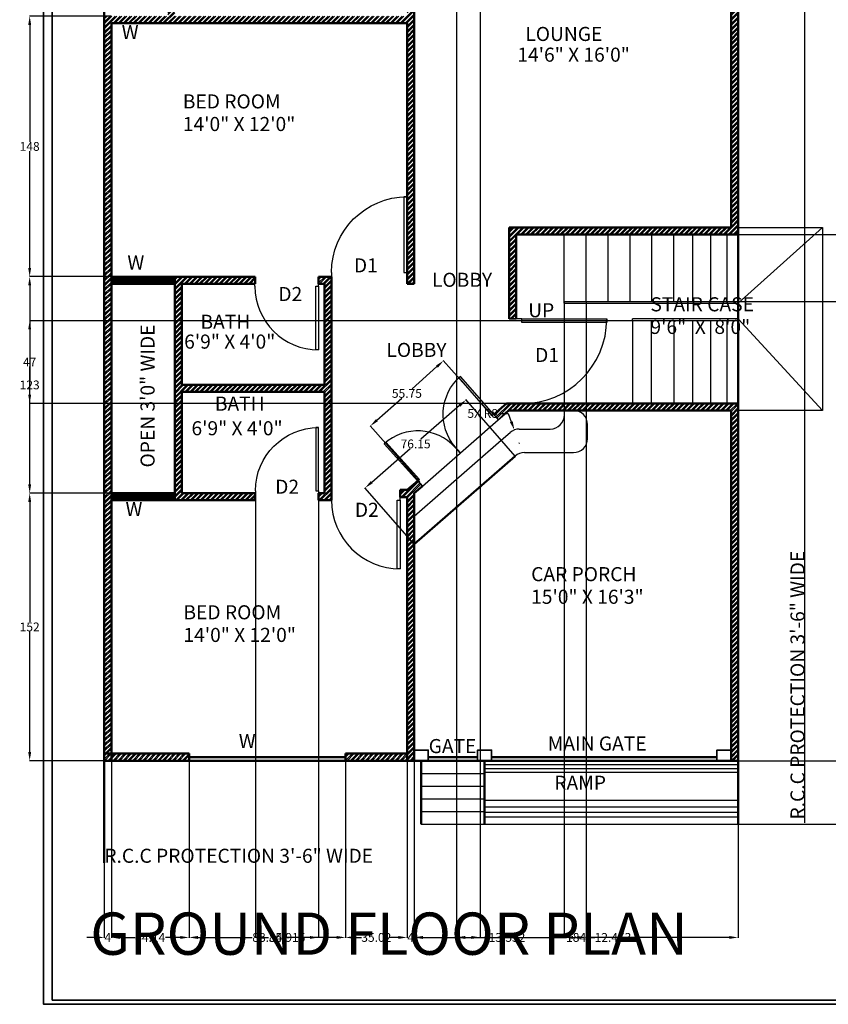
# Model space of a CAD drawing. Units: inches. Extents: x -35 to 905, y -602 to 298.
# Tile 1 of 4: x -30 to 429, y -602 to -43. Entities that reach past the tile are written whole.
import ezdxf

# ---------------------------------------------------------------- set-up
doc = ezdxf.new("R2010")
doc.units = ezdxf.units.IN
doc.header["$MEASUREMENT"] = 0
for name, color, linetype, lineweight in [('A-ANNO-DIMS', 2, 'Continuous', 18), ('A-ANNO-TEXT', 3, 'Continuous', 18), ('A-ANNO-TTLB', 7, 'Continuous', 35), ('A-AREA-IDEN', 7, 'Continuous', 18), ('A-COLS', 7, 'Continuous', 35), ('A-DOOR', 4, 'Continuous', 25), ('A-FLOR-STRS', 3, 'Continuous', 25), ('A-WALL', 7, 'Continuous', 50), ('A-WALL-PATT', 8, 'Continuous', 13), ('C-PROP', 1, 'Continuous', 25)]:
    doc.layers.add(name, color=color, linetype=linetype, lineweight=lineweight)
doc.styles.get("Standard").update_dxf_attribs({"font": 'arial.ttf'})
doc.dimstyles.get("Standard").update_dxf_attribs({"dimtxt": 5, "dimasz": 5, "dimexe": 0.18, "dimexo": 0.0625, "dimgap": 0.09, "dimtad": 0, "dimtih": 1, "dimtoh": 1, "dimdec": 1, "dimzin": 0, "dimdsep": 46, "dimlunit": 4, "dimtxsty": 'Standard', "dimcen": 0.09, "dimadec": 0, "dimazin": 0, "dimtfac": 1, "dimtdec": 1, "dimtofl": 0, "dimtmove": 0, "dimatfit": 3, "dimfxl": 1, "dimtolj": 1, "dimtzin": 0, "dimarcsym": 0})

# ---------------------------------------------------------------- blocks, each defined once
blk = doc.blocks.new('*U2')
for p, q in [((0, 0), (0, -6)), ((40, 0), (40, -6))]:
    blk.add_line(p, q)
blk.add_lwpolyline([(0, 0), (0, 40), (1.75, 40), (1.75, 0)], close=True)
blk.add_arc((0, 0), 40, 0, 90)
blk = doc.blocks.new('*D8')
at = {"layer": 'A-ANNO-DIMS', "color": 0, "lineweight": -2, "ltscale": 0.3, "transparency": 16777216}
for p, q in [((21.72, -40.65), (-24.8, -40.65)), ((-24.62, -45.65), (-24.62, -112.01)), ((-24.62, -183.65), (-24.62, -117.3)), ((21.72, -188.65), (-24.8, -188.65))]:
    blk.add_line(p, q, dxfattribs=at)
at = {"layer": 'A-ANNO-DIMS', "color": 0, "ltscale": 0.3, "transparency": 16777216}
for points in [[(-25.45, -45.65), (-23.78, -45.65), (-24.62, -40.65)], [(-25.45, -183.65), (-23.78, -183.65), (-24.62, -188.65)]]:
    blk.add_solid(points, dxfattribs=at)
at = {"layer": 'Defpoints', "color": 0, "ltscale": 0.3, "transparency": 16777216}
for p in [(21.78, -40.65), (-24.62, -188.65), (21.78, -188.65)]:
    blk.add_point(p, dxfattribs=at)
at = {"layer": 'A-ANNO-DIMS', "color": 0, "ltscale": 0.3, "transparency": 16777216, "insert": (-24.62, -114.65), "char_height": 5, "attachment_point": 5}
blk.add_mtext('\\A1;148', dxfattribs=at)
blk = doc.blocks.new('*D9')
at = {"layer": 'A-ANNO-DIMS', "color": 0, "lineweight": -2, "ltscale": 0.3, "transparency": 16777216}
for p, q in [((21.72, -188.65), (-24.8, -188.65)), ((-24.62, -193.65), (-24.62, -247.51)), ((-24.62, -306.65), (-24.62, -252.8)), ((21.72, -311.65), (-24.8, -311.65))]:
    blk.add_line(p, q, dxfattribs=at)
at = {"layer": 'A-ANNO-DIMS', "color": 0, "ltscale": 0.3, "transparency": 16777216}
for points in [[(-25.45, -193.65), (-23.78, -193.65), (-24.62, -188.65)], [(-25.45, -306.65), (-23.78, -306.65), (-24.62, -311.65)]]:
    blk.add_solid(points, dxfattribs=at)
at = {"layer": 'Defpoints', "color": 0, "ltscale": 0.3, "transparency": 16777216}
for p in [(21.78, -188.65), (-24.62, -311.65), (21.78, -311.65)]:
    blk.add_point(p, dxfattribs=at)
at = {"layer": 'A-ANNO-DIMS', "color": 0, "ltscale": 0.3, "transparency": 16777216, "insert": (-24.62, -250.15), "char_height": 5, "attachment_point": 5}
blk.add_mtext('\\A1;123', dxfattribs=at)
blk = doc.blocks.new('*D10')
at = {"layer": 'A-ANNO-DIMS', "color": 0, "lineweight": -2, "ltscale": 0.3, "transparency": 16777216}
for p, q in [((21.72, -311.65), (-24.8, -311.65)), ((-24.62, -316.65), (-24.62, -385.01)), ((-24.62, -458.65), (-24.62, -390.3)), ((17.72, -463.65), (-24.8, -463.65))]:
    blk.add_line(p, q, dxfattribs=at)
at = {"layer": 'A-ANNO-DIMS', "color": 0, "ltscale": 0.3, "transparency": 16777216}
for points in [[(-25.45, -316.65), (-23.78, -316.65), (-24.62, -311.65)], [(-25.45, -458.65), (-23.78, -458.65), (-24.62, -463.65)]]:
    blk.add_solid(points, dxfattribs=at)
at = {"layer": 'Defpoints', "color": 0, "ltscale": 0.3, "transparency": 16777216}
for p in [(21.78, -311.65), (-24.62, -463.65), (17.78, -463.65)]:
    blk.add_point(p, dxfattribs=at)
at = {"layer": 'A-ANNO-DIMS', "color": 0, "ltscale": 0.3, "transparency": 16777216, "insert": (-24.62, -387.65), "char_height": 5, "attachment_point": 5}
blk.add_mtext('\\A1;152', dxfattribs=at)
blk = doc.blocks.new('*D11')
at = {"layer": 'A-ANNO-DIMS', "color": 0, "lineweight": -2, "ltscale": 0.3, "transparency": 16777216}
for p, q in [((17.78, -463.72), (17.78, -564.24)), ((21.78, -463.72), (21.78, -564.24)), ((12.78, -564.06), (7.78, -564.06)), ((26.78, -564.06), (31.78, -564.06))]:
    blk.add_line(p, q, dxfattribs=at)
at = {"layer": 'A-ANNO-DIMS', "color": 0, "ltscale": 0.3, "transparency": 16777216}
for points in [[(12.78, -563.23), (12.78, -564.9), (17.78, -564.06)], [(26.78, -563.23), (26.78, -564.9), (21.78, -564.06)]]:
    blk.add_solid(points, dxfattribs=at)
at = {"layer": 'Defpoints', "color": 0, "ltscale": 0.3, "transparency": 16777216}
for p in [(17.78, -463.65), (21.78, -463.65), (21.78, -564.06)]:
    blk.add_point(p, dxfattribs=at)
at = {"layer": 'A-ANNO-DIMS', "color": 0, "ltscale": 0.3, "transparency": 16777216, "insert": (19.78, -564.06), "char_height": 5, "attachment_point": 5}
blk.add_mtext('\\A1;4', dxfattribs=at)
blk = doc.blocks.new('*D12')
at = {"layer": 'A-ANNO-DIMS', "color": 0, "lineweight": -2, "ltscale": 0.3, "transparency": 16777216}
for p, q in [((21.78, -463.72), (21.78, -564.24)), ((65.92, -459.72), (65.92, -564.24)), ((26.78, -564.06), (35.24, -564.06)), ((60.92, -564.06), (52.47, -564.06))]:
    blk.add_line(p, q, dxfattribs=at)
at = {"layer": 'A-ANNO-DIMS', "color": 0, "ltscale": 0.3, "transparency": 16777216}
for points in [[(26.78, -563.23), (26.78, -564.9), (21.78, -564.06)], [(60.92, -563.23), (60.92, -564.9), (65.92, -564.06)]]:
    blk.add_solid(points, dxfattribs=at)
at = {"layer": 'Defpoints', "color": 0, "ltscale": 0.3, "transparency": 16777216}
for p in [(21.78, -463.65), (65.92, -459.65), (65.92, -564.06)]:
    blk.add_point(p, dxfattribs=at)
at = {"layer": 'A-ANNO-DIMS', "color": 0, "ltscale": 0.3, "transparency": 16777216, "insert": (43.85, -564.06), "char_height": 5, "attachment_point": 5}
blk.add_mtext('\\A1;44.14', dxfattribs=at)
blk = doc.blocks.new('*D13')
at = {"layer": 'A-ANNO-DIMS', "color": 0, "lineweight": -2, "ltscale": 0.3, "transparency": 16777216}
for p, q in [((65.92, -459.72), (65.92, -564.24)), ((154.77, -459.72), (154.77, -564.24)), ((70.92, -564.06), (101.83, -564.06)), ((149.77, -564.06), (118.86, -564.06))]:
    blk.add_line(p, q, dxfattribs=at)
at = {"layer": 'A-ANNO-DIMS', "color": 0, "ltscale": 0.3, "transparency": 16777216}
for points in [[(70.92, -563.23), (70.92, -564.9), (65.92, -564.06)], [(149.77, -563.23), (149.77, -564.9), (154.77, -564.06)]]:
    blk.add_solid(points, dxfattribs=at)
at = {"layer": 'Defpoints', "color": 0, "ltscale": 0.3, "transparency": 16777216}
for p in [(65.92, -459.65), (154.77, -459.65), (154.77, -564.06)]:
    blk.add_point(p, dxfattribs=at)
at = {"layer": 'A-ANNO-DIMS', "color": 0, "ltscale": 0.3, "transparency": 16777216, "insert": (110.35, -564.06), "char_height": 5, "attachment_point": 5}
blk.add_mtext('\\A1;88.84', dxfattribs=at)
blk = doc.blocks.new('*D14')
at = {"layer": 'A-ANNO-DIMS', "color": 0, "lineweight": -2, "ltscale": 0.3, "transparency": 16777216}
for p, q in [((154.77, -459.72), (154.77, -564.24)), ((189.78, -459.72), (189.78, -564.24)), ((159.77, -564.06), (163.78, -564.06)), ((184.78, -564.06), (180.77, -564.06))]:
    blk.add_line(p, q, dxfattribs=at)
at = {"layer": 'A-ANNO-DIMS', "color": 0, "ltscale": 0.3, "transparency": 16777216}
for points in [[(159.77, -563.23), (159.77, -564.9), (154.77, -564.06)], [(184.78, -563.23), (184.78, -564.9), (189.78, -564.06)]]:
    blk.add_solid(points, dxfattribs=at)
at = {"layer": 'Defpoints', "color": 0, "ltscale": 0.3, "transparency": 16777216}
for p in [(154.77, -459.65), (189.78, -459.65), (189.78, -564.06)]:
    blk.add_point(p, dxfattribs=at)
at = {"layer": 'A-ANNO-DIMS', "color": 0, "ltscale": 0.3, "transparency": 16777216, "insert": (172.28, -564.06), "char_height": 5, "attachment_point": 5}
blk.add_mtext('\\A1;35.02', dxfattribs=at)
blk = doc.blocks.new('*D15')
at = {"layer": 'A-ANNO-DIMS', "color": 0, "lineweight": -2, "ltscale": 0.3, "transparency": 16777216}
for p, q in [((193.78, -457.67), (193.78, -564.24)), ((189.78, -459.72), (189.78, -564.24)), ((184.78, -564.06), (179.78, -564.06)), ((198.78, -564.06), (203.78, -564.06))]:
    blk.add_line(p, q, dxfattribs=at)
at = {"layer": 'A-ANNO-DIMS', "color": 0, "ltscale": 0.3, "transparency": 16777216}
for points in [[(184.78, -563.23), (184.78, -564.9), (189.78, -564.06)], [(198.78, -563.23), (198.78, -564.9), (193.78, -564.06)]]:
    blk.add_solid(points, dxfattribs=at)
at = {"layer": 'Defpoints', "color": 0, "ltscale": 0.3, "transparency": 16777216}
for p in [(193.78, -457.61), (189.78, -459.65), (193.78, -564.06)]:
    blk.add_point(p, dxfattribs=at)
at = {"layer": 'A-ANNO-DIMS', "color": 0, "ltscale": 0.3, "transparency": 16777216, "insert": (191.78, -564.06), "char_height": 5, "attachment_point": 5}
blk.add_mtext('\\A1;4', dxfattribs=at)
blk = doc.blocks.new('*D16')
at = {"layer": 'A-ANNO-DIMS', "color": 0, "lineweight": -2, "ltscale": 0.3, "transparency": 16777216}
for p, q in [((193.78, -457.67), (193.78, -564.24)), ((377.78, -463.72), (377.78, -564.24)), ((198.78, -564.06), (280.42, -564.06)), ((372.78, -564.06), (291.15, -564.06))]:
    blk.add_line(p, q, dxfattribs=at)
at = {"layer": 'A-ANNO-DIMS', "color": 0, "ltscale": 0.3, "transparency": 16777216}
for points in [[(198.78, -563.23), (198.78, -564.9), (193.78, -564.06)], [(372.78, -563.23), (372.78, -564.9), (377.78, -564.06)]]:
    blk.add_solid(points, dxfattribs=at)
at = {"layer": 'Defpoints', "color": 0, "ltscale": 0.3, "transparency": 16777216}
for p in [(193.78, -457.61), (377.78, -463.65), (377.78, -564.06)]:
    blk.add_point(p, dxfattribs=at)
at = {"layer": 'A-ANNO-DIMS', "color": 0, "ltscale": 0.3, "transparency": 16777216, "insert": (285.78, -564.06), "char_height": 5, "attachment_point": 5}
blk.add_mtext('\\A1;184', dxfattribs=at)
blk = doc.blocks.new('*D17')
at = {"layer": 'A-ANNO-DIMS', "color": 0, "lineweight": -2, "ltscale": 0.3, "transparency": 16777216}
for p, q in [((377.85, -463.65), (468.36, -463.65)), ((468.18, -468.65), (468.18, -479.01)), ((468.18, -494.65), (468.18, -484.3)), ((377.85, -499.65), (468.36, -499.65))]:
    blk.add_line(p, q, dxfattribs=at)
at = {"layer": 'A-ANNO-DIMS', "color": 0, "ltscale": 0.3, "transparency": 16777216}
for points in [[(467.35, -468.65), (469.02, -468.65), (468.18, -463.65)], [(467.35, -494.65), (469.02, -494.65), (468.18, -499.65)]]:
    blk.add_solid(points, dxfattribs=at)
at = {"layer": 'Defpoints', "color": 0, "ltscale": 0.3, "transparency": 16777216}
for p in [(377.78, -463.65), (377.78, -499.65), (468.18, -499.65)]:
    blk.add_point(p, dxfattribs=at)
at = {"layer": 'A-ANNO-DIMS', "color": 0, "ltscale": 0.3, "transparency": 16777216, "insert": (468.18, -481.65), "char_height": 5, "attachment_point": 5}
blk.add_mtext('\\A1;36', dxfattribs=at)
blk = doc.blocks.new('*D18')
at = {"layer": 'A-ANNO-DIMS', "color": 0, "lineweight": -2, "ltscale": 0.3, "transparency": 16777216}
for p, q in [((377.85, 249.35), (468.36, 249.35)), ((468.18, 244.35), (468.18, -104.51)), ((468.18, -458.65), (468.18, -109.8)), ((377.85, -463.65), (468.36, -463.65))]:
    blk.add_line(p, q, dxfattribs=at)
at = {"layer": 'A-ANNO-DIMS', "color": 0, "ltscale": 0.3, "transparency": 16777216}
for points in [[(467.35, 244.35), (469.02, 244.35), (468.18, 249.35)], [(467.35, -458.65), (469.02, -458.65), (468.18, -463.65)]]:
    blk.add_solid(points, dxfattribs=at)
at = {"layer": 'Defpoints', "color": 0, "ltscale": 0.3, "transparency": 16777216}
for p in [(377.78, 249.35), (377.78, -463.65), (468.18, -463.65)]:
    blk.add_point(p, dxfattribs=at)
at = {"layer": 'A-ANNO-DIMS', "color": 0, "ltscale": 0.3, "transparency": 16777216, "insert": (468.18, -107.15), "char_height": 5, "attachment_point": 5}
blk.add_mtext('\\A1;713', dxfattribs=at)
blk = doc.blocks.new('*D21')
at = {"layer": 'A-ANNO-DIMS', "color": 0, "lineweight": -2, "ltscale": 0.3, "transparency": 16777216}
for p, q in [((103.62, -315.72), (103.62, -564.24)), ((139.54, -315.72), (139.54, -564.24)), ((108.62, -564.06), (111.09, -564.06)), ((134.54, -564.06), (132.07, -564.06))]:
    blk.add_line(p, q, dxfattribs=at)
at = {"layer": 'A-ANNO-DIMS', "color": 0, "ltscale": 0.3, "transparency": 16777216}
for points in [[(108.62, -563.23), (108.62, -564.9), (103.62, -564.06)], [(134.54, -563.23), (134.54, -564.9), (139.54, -564.06)]]:
    blk.add_solid(points, dxfattribs=at)
at = {"layer": 'Defpoints', "color": 0, "ltscale": 0.3, "transparency": 16777216}
for p in [(103.62, -315.65), (139.54, -315.65), (139.54, -564.06)]:
    blk.add_point(p, dxfattribs=at)
at = {"layer": 'A-ANNO-DIMS', "color": 0, "ltscale": 0.3, "transparency": 16777216, "insert": (121.58, -564.06), "char_height": 5, "attachment_point": 5}
blk.add_mtext('\\A1;35.915', dxfattribs=at)
blk = doc.blocks.new('*D24')
at = {"layer": 'A-ANNO-DIMS', "color": 0, "lineweight": -2, "ltscale": 0.3, "transparency": 16777216}
for p, q in [((206.74, -239.75), (192.62, -252.35)), ((238.65, -268.02), (210.35, -236.29)), ((172.6, -270.21), (186.72, -257.61)), ((197.05, -305.13), (168.75, -273.4))]:
    blk.add_line(p, q, dxfattribs=at)
at = {"layer": 'A-ANNO-DIMS', "color": 0, "ltscale": 0.3, "transparency": 16777216}
for points in [[(206.18, -239.13), (207.29, -240.37), (210.47, -236.42)], [(172.05, -269.58), (173.16, -270.83), (168.87, -273.54)]]:
    blk.add_solid(points, dxfattribs=at)
at = {"layer": 'Defpoints', "color": 0, "ltscale": 0.3, "transparency": 16777216}
for p in [(210.47, -236.42), (238.7, -268.06), (197.1, -305.17)]:
    blk.add_point(p, dxfattribs=at)
at = {"layer": 'A-ANNO-DIMS', "color": 0, "ltscale": 0.3, "transparency": 16777216, "insert": (189.67, -254.98), "char_height": 5, "attachment_point": 5}
blk.add_mtext('\\A1;55.75', dxfattribs=at)
blk = doc.blocks.new('*D25')
at = {"layer": 'A-ANNO-DIMS', "color": 0, "lineweight": -2, "ltscale": 0.3, "transparency": 16777216}
for p, q in [((217.78, 218.55), (217.78, -564.24)), ((231.32, 218.55), (231.32, -564.24)), ((222.78, -564.06), (226.32, -564.06)), ((231.32, -564.06), (236.32, -564.06))]:
    blk.add_line(p, q, dxfattribs=at)
at = {"layer": 'A-ANNO-DIMS', "color": 0, "ltscale": 0.3, "transparency": 16777216}
for points in [[(222.78, -563.23), (222.78, -564.9), (217.78, -564.06)], [(226.32, -563.23), (226.32, -564.9), (231.32, -564.06)]]:
    blk.add_solid(points, dxfattribs=at)
at = {"layer": 'Defpoints', "color": 0, "ltscale": 0.3, "transparency": 16777216}
for p in [(217.78, 218.61), (231.32, 218.61), (231.32, -564.06)]:
    blk.add_point(p, dxfattribs=at)
at = {"layer": 'A-ANNO-DIMS', "color": 0, "ltscale": 0.3, "transparency": 16777216, "insert": (246.52, -564.06), "char_height": 5, "attachment_point": 5}
blk.add_mtext('\\A1;13.532', dxfattribs=at)
blk = doc.blocks.new('*D27')
at = {"layer": 'A-ANNO-DIMS', "color": 0, "lineweight": -2, "ltscale": 0.3, "transparency": 16777216}
for p, q in [((279.03, -202.74), (279.03, -564.24)), ((291.5, -202.74), (291.5, -564.24)), ((284.03, -564.06), (286.5, -564.06)), ((291.5, -564.06), (296.5, -564.06))]:
    blk.add_line(p, q, dxfattribs=at)
at = {"layer": 'A-ANNO-DIMS', "color": 0, "ltscale": 0.3, "transparency": 16777216}
for points in [[(284.03, -563.23), (284.03, -564.9), (279.03, -564.06)], [(286.5, -563.23), (286.5, -564.9), (291.5, -564.06)]]:
    blk.add_solid(points, dxfattribs=at)
at = {"layer": 'Defpoints', "color": 0, "ltscale": 0.3, "transparency": 16777216}
for p in [(279.03, -202.67), (291.5, -202.67), (291.5, -564.06)]:
    blk.add_point(p, dxfattribs=at)
at = {"layer": 'A-ANNO-DIMS', "color": 0, "ltscale": 0.3, "transparency": 16777216, "insert": (306.73, -564.06), "char_height": 5, "attachment_point": 5}
blk.add_mtext('\\A1;12.463', dxfattribs=at)
blk = doc.blocks.new('*D28')
at = {"layer": 'A-ANNO-DIMS', "color": 0, "lineweight": -2, "ltscale": 0.3, "transparency": 16777216}
for p, q in [((279.1, -164.65), (468.36, -164.65)), ((468.18, -169.65), (468.18, -181.02)), ((468.18, -197.67), (468.18, -186.31)), ((279.1, -202.67), (468.36, -202.67))]:
    blk.add_line(p, q, dxfattribs=at)
at = {"layer": 'A-ANNO-DIMS', "color": 0, "ltscale": 0.3, "transparency": 16777216}
for points in [[(467.35, -169.65), (469.02, -169.65), (468.18, -164.65)], [(467.35, -197.67), (469.02, -197.67), (468.18, -202.67)]]:
    blk.add_solid(points, dxfattribs=at)
at = {"layer": 'Defpoints', "color": 0, "ltscale": 0.3, "transparency": 16777216}
for p in [(279.03, -164.65), (279.03, -202.67), (468.18, -202.67)]:
    blk.add_point(p, dxfattribs=at)
at = {"layer": 'A-ANNO-DIMS', "color": 0, "ltscale": 0.3, "transparency": 16777216, "insert": (468.18, -183.66), "char_height": 5, "attachment_point": 5}
blk.add_mtext('\\A1;38.02', dxfattribs=at)
blk = doc.blocks.new('*D29')
at = {"layer": 'A-ANNO-DIMS', "color": 0, "lineweight": -2, "ltscale": 0.3, "transparency": 16777216}
for p, q in [((317.72, -213.65), (-24.8, -213.65)), ((-24.62, -218.65), (-24.62, -234.56)), ((-24.62, -255.65), (-24.62, -239.74)), ((317.72, -260.65), (-24.8, -260.65))]:
    blk.add_line(p, q, dxfattribs=at)
at = {"layer": 'A-ANNO-DIMS', "color": 0, "ltscale": 0.3, "transparency": 16777216}
for points in [[(-25.45, -218.65), (-23.78, -218.65), (-24.62, -213.65)], [(-25.45, -255.65), (-23.78, -255.65), (-24.62, -260.65)]]:
    blk.add_solid(points, dxfattribs=at)
at = {"layer": 'Defpoints', "color": 0, "ltscale": 0.3, "transparency": 16777216}
for p in [(317.78, -213.65), (-24.62, -260.65), (317.78, -260.65)]:
    blk.add_point(p, dxfattribs=at)
at = {"layer": 'A-ANNO-DIMS', "color": 0, "ltscale": 0.3, "transparency": 16777216, "insert": (-24.62, -237.15), "char_height": 5, "attachment_point": 5}
blk.add_mtext('\\A1;47', dxfattribs=at)
blk = doc.blocks.new('*D30')
at = {"layer": 'A-ANNO-DIMS', "color": 0, "lineweight": -2, "ltscale": 0.3, "transparency": 16777216}
for p, q in [((219.53, -261.92), (197.63, -281.03)), ((251.13, -290.54), (223.18, -258.5)), ((169.68, -305.41), (191.57, -286.31)), ((193.74, -340.6), (165.79, -308.57))]:
    blk.add_line(p, q, dxfattribs=at)
at = {"layer": 'A-ANNO-DIMS', "color": 0, "ltscale": 0.3, "transparency": 16777216}
for points in [[(218.98, -261.3), (220.07, -262.55), (223.29, -258.64)], [(169.13, -304.79), (170.23, -306.04), (165.91, -308.7)]]:
    blk.add_solid(points, dxfattribs=at)
at = {"layer": 'Defpoints', "color": 0, "ltscale": 0.3, "transparency": 16777216}
for p in [(223.29, -258.64), (251.17, -290.59), (193.78, -340.65)]:
    blk.add_point(p, dxfattribs=at)
at = {"layer": 'A-ANNO-DIMS', "color": 0, "ltscale": 0.3, "transparency": 16777216, "insert": (194.6, -283.67), "char_height": 5, "attachment_point": 5}
blk.add_mtext('\\A1;76.15', dxfattribs=at)
blk = doc.blocks.new('*D58')
at = {"layer": 'A-ANNO-DIMS', "color": 0, "lineweight": -2, "ltscale": 0.3, "transparency": 16777216}
for p, q in [((242.21, -266.36), (247.21, -266.36)), ((247.21, -266.36), (248.97, -271.04)), ((253.44, -283.22), (253.62, -283.22)), ((253.53, -283.31), (253.53, -283.13))]:
    blk.add_line(p, q, dxfattribs=at)
at = {"layer": 'A-ANNO-DIMS', "color": 0, "ltscale": 0.3, "transparency": 16777216}
blk.add_solid([(249.75, -270.75), (248.19, -271.34), (250.72, -275.73)], dxfattribs=at)
at = {"layer": 'Defpoints', "color": 0, "ltscale": 0.3, "transparency": 16777216}
for p in [(250.72, -275.73), (253.53, -283.22)]:
    blk.add_point(p, dxfattribs=at)
at = {"layer": 'A-ANNO-DIMS', "color": 0, "ltscale": 0.3, "transparency": 16777216, "insert": (232.71, -266.36), "char_height": 5, "attachment_point": 5}
blk.add_mtext('\\A1;5X R8', dxfattribs=at)

msp = doc.modelspace()

# ---------------------------------------------------------------- hatches: boundary and pattern name
at = {"layer": 'A-WALL-PATT', "ltscale": 0.3}
h = msp.add_hatch(dxfattribs=at)
h.set_pattern_fill('ANSI32', color=256, scale=5.3)
h.paths.add_polyline_path([(103.5369, -188.6534), (57.7847, -188.6534), (57.7847, -315.6534), (103.5369, -315.6534), (103.5369, -311.6534), (61.7847, -311.6534), (61.7847, -254.1534), (142.7847, -254.1534), (142.7847, -311.6534), (139.5369, -311.6534), (139.5369, -315.6534), (146.7847, -315.6534), (146.7847, -250.1534), (146.7847, -188.6534), (139.5369, -188.6534), (139.5369, -192.6534), (142.7847, -192.6534), (142.7847, -250.1534), (61.7847, -250.1534), (61.7847, -192.6534), (103.5369, -192.6534)], flags=17)
h.paths.add_polyline_path([(251.7847, -164.6534), (377.7847, -164.6534), (377.7847, 107.3466), (377.7847, 249.3466), (55.7847, 249.3466), (55.7847, 167.3466), (189.7847, 167.3466), (189.7847, 79.3466), (193.7847, 79.3466), (193.7847, 107.3466), (199.7871, 107.3466), (199.7871, 111.3466), (193.7847, 111.3466), (193.7847, 177.7106), (189.7847, 177.7106), (189.7847, 171.3466), (105.7847, 171.3466), (105.7847, 177.7106), (101.7847, 177.7106), (101.7847, 171.3466), (59.7847, 171.3466), (59.7847, 243.3466), (101.7847, 243.3466), (101.7847, 201.7106), (105.7847, 201.7106), (105.7847, 243.3466), (189.7847, 243.3466), (189.7847, 213.7106), (193.7847, 213.7106), (193.7847, 243.3466), (375.7847, 243.3466), (375.7847, 111.3466), (255.7847, 111.3466), (255.7847, 81.4115), (259.7847, 81.4115), (259.7847, 107.3466), (373.7847, 107.3466), (373.7847, 35.3466), (255.7847, 35.3466), (255.7847, 31.3466), (373.7847, 31.3466), (373.7847, -160.6534), (247.7847, -160.6534), (247.7847, -164.6534), (247.7847, -212.6534), (251.7847, -212.6534)])
h.paths.add_polyline_path([(193.7847, -311.6534), (198.4452, -307.597), (195.8191, -304.5798), (189.7847, -309.832), (185.845, -309.832), (185.845, -313.832), (189.7847, -313.832), (189.7847, -463.6534), (193.7847, -463.6534), (193.7847, -457.6052)])
h.paths.add_polyline_path([(377.7847, -260.6534), (246.2878, -260.6534), (238.9641, -267.0277), (241.5902, -270.0449), (247.7847, -264.6534), (373.7847, -264.6534), (373.7847, -463.6534), (377.7847, -463.6534)])
h.paths.add_polyline_path([(189.7847, -459.6534), (154.7661, -459.6534), (154.7661, -463.6534), (189.7847, -463.6534)])
h.paths.add_polyline_path([(65.9248, -459.6534), (21.7847, -459.6534), (21.7847, -463.6534), (65.9248, -463.6534)])
h.paths.add_polyline_path([(21.7847, -459.6534), (17.7847, -459.6534), (17.7847, -463.6534), (21.7847, -463.6534)])
h = msp.add_hatch(dxfattribs=at)
h.set_pattern_fill('ANSI32', color=256, scale=5.3)
h.paths.add_polyline_path([(193.7847, 31.3466), (189.7847, 31.3466), (189.7847, 23.3466), (156.106, 23.3466), (156.106, 19.3466), (189.7847, 19.3466), (189.7847, -40.6534), (57.7847, -40.6534), (57.7847, 19.3466), (120.106, 19.3466), (120.106, 23.3466), (21.7847, 23.3466), (21.7847, 167.3466), (17.7847, 167.3466), (17.7847, 19.3466), (53.7847, 19.3466), (53.7847, -40.6534), (17.7847, -40.6534), (17.7847, -459.6534), (21.7847, -459.6534), (21.7847, -315.6534), (21.7847, -192.6534), (21.7847, -44.6534), (189.7847, -44.6534), (189.7847, -188.6534), (189.7847, -192.6534), (193.7847, -192.6534)])

# ---------------------------------------------------------------- linework, layer by layer
at = {"layer": 'A-ANNO-TTLB', "ltscale": 0.3}
for points in [[(-16.7606, 298.2205), (890.3824, 298.2205), (890.3824, -602.0527), (-16.7606, -602.0527)], [(-11.7606, 293.2205), (885.3824, 293.2205), (885.3824, -599.6301), (-11.7606, -599.6301)]]:
    msp.add_lwpolyline(points, close=True, dxfattribs=at)
at = {"layer": 'A-COLS'}
for points in [[(193.7847, -463.6534), (201.7701, -463.6534), (201.7701, -457.6052), (193.7847, -457.6052)], [(229.8055, -463.6534), (237.7909, -463.6534), (237.7909, -457.6052), (229.8055, -457.6052)], [(365.7993, -463.6534), (373.7847, -463.6534), (373.7847, -457.6052), (365.7993, -457.6052)]]:
    msp.add_lwpolyline(points, close=True, dxfattribs=at)
at = {"layer": 'A-FLOR-STRS', "ltscale": 0.3}
for p, q in [((377.7847, -160.6534), (425.7847, -160.6534)), ((377.7847, -203.6738), (425.7847, -160.6534)), ((425.7847, -160.6534), (425.7847, -264.6534)), ((279.0335, -202.6738), (279.0335, -164.6534)), ((291.4969, -202.6738), (291.4969, -164.6534)), ((303.9603, -202.6738), (303.9603, -164.6534)), ((316.4237, -202.6738), (316.4237, -164.6534)), ((328.8871, -202.6738), (328.8871, -164.6534)), ((341.3505, -202.6738), (341.3505, -164.6534)), ((341.3505, -202.6738), (341.3505, -164.6534)), ((351.8132, -164.6534), (351.8132, -202.6738)), ((362.0945, -164.6534), (362.0945, -202.6738)), ((371.3335, -164.6534), (371.3335, -202.6738)), ((279.0335, -202.6738), (377.7847, -202.6738)), ((279.0335, -203.6738), (279.0335, -202.6738)), ((279.0335, -203.6738), (377.7847, -203.6738)), ((377.7847, -203.6738), (377.7847, -212.6534)), ((377.7847, -212.6534), (317.7847, -212.6534)), ((317.7847, -213.6534), (317.7847, -212.6534)), ((377.7847, -213.6534), (317.7847, -213.6534)), ((317.7847, -213.6534), (317.7847, -260.6534)), ((328.4091, -213.6534), (328.4091, -260.6534)), ((341.3505, -213.6534), (341.3505, -260.6534)), ((351.8132, -213.6534), (351.8132, -260.6534)), ((362.0945, -213.6534), (362.0945, -260.6534)), ((371.3335, -213.6534), (371.3335, -260.6534)), ((377.7847, -212.6534), (425.7847, -264.6534)), ((279.1164, -267.2171), (279.1164, -264.6534)), ((425.7847, -264.6534), (377.7847, -264.6534)), ((243.2794, -281.5447), (248.2722, -277.1889)), ((253.5315, -275.2171), (271.1164, -275.2171)), ((193.7847, -324.7257), (243.2794, -281.5447)), ((233.7982, -465.8032), (377.7847, -465.8032)), ((233.7982, -468.1653), (377.7847, -468.1653)), ((197.7774, -470.8534), (233.7982, -470.8534)), ((233.7982, -470.1104), (377.7847, -470.1104)), ((197.7774, -478.0534), (233.7982, -478.0534)), ((197.7774, -485.2534), (233.7982, -485.2534)), ((233.7982, -486.1006), (377.7847, -486.1006)), ((233.7982, -489.7952), (377.7847, -489.7952)), ((197.7774, -492.4534), (233.7982, -492.4534)), ((233.7982, -492.9435), (377.7847, -492.9435)), ((233.7982, -495.4534), (377.7847, -495.4534)), ((197.7774, -499.6534), (233.7982, -499.6534)), ((233.7982, -499.6534), (377.7847, -499.6534))]:
    msp.add_line(p, q, dxfattribs=at)
at = {"layer": 'A-FLOR-STRS'}
for p, q in [((247.7847, -212.6534), (251.7847, -212.6534)), ((238.9641, -267.0277), (241.5902, -270.0449)), ((241.5902, -270.0449), (247.7847, -264.6534)), ((195.8191, -304.5798), (198.4452, -307.597))]:
    msp.add_line(p, q, dxfattribs=at)
at = {"layer": 'A-FLOR-STRS', "ltscale": 0.3}
msp.add_lwpolyline([(256.4276, -288.6154), (284.3001, -288.6154, 0.41421356), (292.3001, -280.6154), (292.3001, -272.6534, 0.41421356), (284.3001, -264.6534), (247.7847, -264.6534)], format="xyb", dxfattribs=at)
msp.add_lwpolyline([(198.4452, -307.597), (241.5902, -270.0449)], dxfattribs=at)
for centre, start, end in [((271.1164, -267.2171), 270, 0), ((253.5315, -283.2171), 90, 131.102607), ((256.4276, -296.6154), 90, 131.102607)]:
    msp.add_arc(centre, 8, start, end, dxfattribs=at)
at = {"layer": 'A-WALL'}
for p, q in [((17.7847, 249.3466), (17.7847, -463.6534)), ((377.7847, 107.3466), (377.7847, -164.6534)), ((193.7847, 31.3466), (193.7847, -192.6534)), ((373.7847, 31.3466), (373.7847, -160.6534)), ((21.7847, -44.6534), (189.7847, -44.6534)), ((21.7847, -44.6534), (21.7847, -192.6534)), ((189.7847, -44.6534), (189.7847, -188.6534)), ((247.7847, -160.6534), (373.7847, -160.6534)), ((247.7847, -160.6534), (247.7847, -164.6534)), ((247.7847, -164.6534), (247.7847, -212.6534)), ((251.7847, -164.6534), (377.7847, -164.6534)), ((251.7847, -212.6534), (251.7847, -164.6534)), ((21.7847, -188.6534), (103.5369, -188.6534)), ((21.7847, -189.6051), (57.7847, -189.6051)), ((57.7847, -188.6534), (57.7847, -315.6534)), ((103.5369, -188.6534), (103.5369, -192.6534)), ((139.5369, -192.6534), (139.5369, -188.6534)), ((139.5369, -188.6534), (146.7847, -188.6534)), ((146.7847, -188.6534), (146.7847, -250.1534)), ((189.7847, -188.6534), (189.7847, -192.6534)), ((21.7847, -190.8554), (57.7847, -190.8554)), ((21.7847, -191.7877), (57.7847, -191.7877)), ((21.7847, -192.6534), (57.7847, -192.6534)), ((21.7847, -192.6534), (21.7847, -315.6534)), ((61.7847, -192.6534), (61.7847, -250.1534)), ((61.7847, -192.6534), (103.5369, -192.6534)), ((139.5369, -192.6534), (142.7847, -192.6534)), ((142.7847, -192.6534), (142.7847, -250.1534)), ((189.7847, -192.6534), (193.7847, -192.6534)), ((61.7847, -250.1534), (142.7847, -250.1534)), ((146.7847, -250.1534), (146.7847, -315.6534)), ((61.7847, -254.1534), (61.7847, -311.6534)), ((61.7847, -254.1534), (142.7847, -254.1534)), ((142.7847, -254.1534), (142.7847, -311.6534)), ((238.9641, -267.0277), (246.2878, -260.6534)), ((246.2878, -260.6534), (377.7847, -260.6534)), ((377.7847, -260.6534), (377.7847, -463.6534)), ((373.7847, -264.6534), (373.7847, -463.6534)), ((189.7847, -309.832), (195.8191, -304.5798)), ((193.7847, -311.6534), (198.4452, -307.597)), ((21.7847, -311.6534), (57.7847, -311.6534)), ((21.7847, -312.3877), (57.7847, -312.3877)), ((61.7847, -311.6534), (103.5369, -311.6534)), ((103.5369, -311.6534), (103.5369, -315.6534)), ((139.5369, -315.6534), (139.5369, -311.6534)), ((139.5369, -311.6534), (142.7847, -311.6534)), ((193.7847, -311.6534), (193.7847, -463.6534)), ((21.7847, -313.638), (57.7847, -313.638)), ((21.7847, -314.5703), (57.7847, -314.5703)), ((21.7847, -315.6534), (103.5369, -315.6534)), ((21.7847, -315.6534), (21.7847, -463.6534)), ((139.5369, -315.6534), (146.7847, -315.6534)), ((189.7847, -313.832), (189.7847, -463.6534)), ((189.7847, -313.832), (189.7847, -315.6534)), ((17.7847, -459.6534), (65.9248, -459.6534)), ((17.7847, -463.6534), (21.7847, -463.6534)), ((21.7847, -463.6534), (189.7847, -463.6534)), ((65.9248, -459.6534), (65.9248, -463.6534)), ((65.9248, -461.6534), (154.7661, -461.6534)), ((154.7661, -459.6534), (154.7661, -463.6534)), ((154.7661, -459.6534), (189.7847, -459.6534)), ((189.7847, -463.6534), (377.7847, -463.6534)), ((201.7701, -461.6534), (229.8055, -461.6534)), ((237.7909, -461.6534), (365.7993, -461.6534))]:
    msp.add_line(p, q, dxfattribs=at)
at = {"layer": 'A-WALL', "ltscale": 0.3}
for p, q in [((377.7847, -164.6534), (377.7847, -260.6534)), ((247.7847, -264.6534), (373.7847, -264.6534)), ((193.7847, -340.6506), (251.1683, -290.5872)), ((189.7847, -309.832), (185.845, -309.832)), ((185.845, -309.832), (185.845, -313.832)), ((185.845, -313.832), (189.7847, -313.832)), ((17.7847, -463.6534), (17.7847, -521.6622)), ((197.7774, -463.6534), (197.7774, -499.6534)), ((197.7774, -463.6534), (233.7982, -463.6534)), ((233.7982, -499.6534), (233.7982, -463.6534)), ((377.7847, -499.6534), (377.7847, -463.6534))]:
    msp.add_line(p, q, dxfattribs=at)
at = {"layer": 'C-PROP', "ltscale": 0.3}
msp.add_line((415.5757, 246.7147), (415.5757, -498.921), dxfattribs=at)

# ---------------------------------------------------------------- block references
at = {"layer": 'A-DOOR'}
for p, xscale, yscale, zscale in [((189.7847, -186.2108), -1.073762759781753, 1.073762759781753, 1.073762759781753), ((139.5013, -310.2715), -0.8969775646550407, 0.8969775646550407, 0.8969775646550407)]:
    msp.add_blockref('*U2', p, dxfattribs=dict(at, xscale=xscale, yscale=yscale, zscale=zscale))
for p, xscale, yscale, zscale, rotation in [((139.5369, -194.078), 0.9041013383372541, 0.9041013383372541, 0.9041013383372541, 180), ((255.0117, -212.6534), 1.204505030704, 1.204505030704, 1.204505030704, 270), ((238.7822, -266.8186), -0.7128608206964421, 0.712860820696442, 0.712860820696442, 41.03534527714415), ((195.9095, -304.7896), 0.7128608206964421, 0.7128608206964421, 0.7128608206964421, 42.02527680153038), ((185.845, -315.6807), 0.9747879651112747, 0.9747879651112747, 0.9747879651112747, 180)]:
    msp.add_blockref('*U2', p, dxfattribs=dict(at, xscale=xscale, yscale=yscale, zscale=zscale, rotation=rotation))

# ---------------------------------------------------------------- texts
at = {"layer": 'A-ANNO-TEXT', "ltscale": 0.3}
for s, height, p in [('W', 8, (27.6499, -53.7175)), ('W', 8, (30.8823, -184.6148)), ('D1', 8, (159.565, -186.2311)), ('D2', 8, (116.6495, -202.5104)), ('UP', 8, (258.5726, -211.7202)), ('D1', 8, (262.4985, -237.1511)), ('D2', 8, (114.8389, -312.0002)), ('W', 8, (29.8304, -324.649)), ('D2', 8, (160.1076, -325.129)), ('W', 8, (94.1627, -456.4558)), ('GATE', 8, (202.0388, -459.3461)), ('MAIN GATE', 8, (269.6716, -457.8921)), ('RAMP', 8, (273.4157, -480.1701)), ('R.C.C PROTECTION 3\'-6" WIDE', 8, (17.7847, -521.6622)), ('GROUND FLOOR PLAN', 24, (9.8083, -573.9217))]:
    msp.add_text(s, height=height, dxfattribs=at).set_placement(p)
msp.add_text('R.C.C PROTECTION 3\'-6" WIDE', height=8, rotation=90, dxfattribs=at).set_placement((415.5757, -497.0688))
at = {"layer": 'A-AREA-IDEN', "ltscale": 0.3}
for s, p in [('LOUNGE', (256.9526, -54.7576)), ('14\'6" X 16\'0"', (252.4156, -66.5276)), ('BED ROOM', (62.3791, -93.0774)), ('14\'0" X 12\'0"', (62.3791, -105.9287)), ('LOBBY', (203.9037, -194.4265)), ('STAIR CASE', (328.0135, -208.3481)), ('BATH', (72.4059, -218.2817)), ('9\'6"  X  8\'0"', (328.0135, -221.1994)), ('6\'9" X 4\'0"', (63.1348, -229.544)), ('LOBBY', (178.0378, -234.2615)), ('BATH', (80.5828, -264.7916)), ('6\'9" X 4\'0"', (67.2852, -278.7555)), ('CAR PORCH', (260.2396, -361.6645)), ('15\'0" X 16\'3"', (260.2396, -374.5158)), ('BED ROOM', (62.7262, -383.333)), ('14\'0" X 12\'0"', (62.7262, -396.1843))]:
    msp.add_text(s, height=8, dxfattribs=at).set_placement(p)
msp.add_text('OPEN 3\'0" WIDE', height=8, rotation=90, dxfattribs=at).set_placement((46.3542, -297.0688))

# ---------------------------------------------------------------- dimensions: what is measured, and where the dimension line sits
at = {"layer": 'A-ANNO-DIMS', "ltscale": 0.3}
for base, p1, p2, angle, override, picture, middle in [((468.1847, -463.6534), (377.7847, 249.3466), (377.7847, -463.6534), 90, {"dimdec": 0, "dimlfac": 1, "dimrnd": 0, "dimzin": 0, "dimdsep": 46, "dimlunit": 2}, '*D18', (468.1847, -107.1534)), ((-24.6153, -188.6534), (21.7847, -40.6534), (21.7847, -188.6534), 90, {"dimdec": 0, "dimlfac": 1, "dimrnd": 0, "dimzin": 0, "dimdsep": 46, "dimlunit": 2}, '*D8', (-24.6153, -114.6534)), ((468.1847, -202.6738), (279.0335, -164.6534), (279.0335, -202.6738), 90, {"dimdec": 2, "dimlfac": 1, "dimrnd": 0, "dimzin": 0, "dimdsep": 46, "dimlunit": 2}, '*D28', (468.1847, -183.6636)), ((-24.6153, -311.6534), (21.7847, -188.6534), (21.7847, -311.6534), 90, {"dimdec": 0, "dimlfac": 1, "dimrnd": 0, "dimzin": 0, "dimdsep": 46, "dimlunit": 2}, '*D9', (-24.6153, -250.1534)), ((-24.6153, -260.6534), (317.7847, -213.6534), (317.7847, -260.6534), 90, {"dimdec": 0, "dimlfac": 1, "dimrnd": 0, "dimzin": 0, "dimdsep": 46, "dimlunit": 2}, '*D29', (-24.6153, -237.1534)), ((210.4701, -236.4236), (197.0961, -305.1746), (238.6959, -268.0631), 41.736355, {"dimdec": 2, "dimlfac": 1, "dimrnd": 0, "dimzin": 0, "dimdsep": 46, "dimlunit": 2}, '*D24', (189.6702, -254.9793)), ((223.2941, -258.6373), (193.7847, -340.6506), (251.1683, -290.5872), 41.102607, {"dimdec": 2, "dimlfac": 1, "dimrnd": 0, "dimzin": 0, "dimdsep": 46, "dimlunit": 2}, '*D30', (194.6023, -283.6691)), ((-24.6153, -463.6534), (21.7847, -311.6534), (17.7847, -463.6534), 90, {"dimdec": 0, "dimlfac": 1, "dimrnd": 0, "dimzin": 0, "dimdsep": 46, "dimlunit": 2}, '*D10', (-24.6153, -387.6534)), ((468.1847, -499.6534), (377.7847, -463.6534), (377.7847, -499.6534), 90, {"dimdec": 0, "dimlfac": 1, "dimrnd": 0, "dimzin": 0, "dimdsep": 46, "dimlunit": 2}, '*D17', (468.1847, -481.6534))]:
    dim = msp.add_linear_dim(base=base, p1=p1, p2=p2, angle=angle, dimstyle='Standard', override=override, dxfattribs=at)
    dim.commit()
    dim.dimension.update_dxf_attribs({"geometry": picture, "text_midpoint": middle})
for base, p1, p2, override, picture, middle in [((231.3167, -564.0622), (217.7847, 218.6126), (231.3167, 218.6126), {"dimdec": 3, "dimlfac": 1, "dimrnd": 0, "dimzin": 0, "dimdsep": 46, "dimlunit": 2}, '*D25', (246.5244, -564.0622)), ((291.4969, -564.0622), (279.0335, -202.6738), (291.4969, -202.6738), {"dimdec": 3, "dimlfac": 1, "dimrnd": 0, "dimzin": 0, "dimdsep": 46, "dimlunit": 2}, '*D27', (306.7301, -564.0622)), ((139.5369, -564.0622), (103.6222, -315.6534), (139.5369, -315.6534), {"dimdec": 3, "dimlfac": 1, "dimrnd": 0, "dimzin": 0, "dimdsep": 46, "dimlunit": 2}, '*D21', (121.5796, -564.0622)), ((193.7847, -564.0622), (189.7847, -459.6534), (193.7847, -457.6052), {"dimdec": 0, "dimlfac": 1, "dimrnd": 0, "dimzin": 0, "dimdsep": 46, "dimlunit": 2}, '*D15', (191.7847, -564.0622)), ((377.7847, -564.0622), (193.7847, -457.6052), (377.7847, -463.6534), {"dimdec": 0, "dimlfac": 1, "dimrnd": 0, "dimzin": 0, "dimdsep": 46, "dimlunit": 2}, '*D16', (285.7847, -564.0622)), ((21.7847, -564.0622), (17.7847, -463.6534), (21.7847, -463.6534), {"dimdec": 0, "dimlfac": 1, "dimrnd": 0, "dimzin": 0, "dimdsep": 46, "dimlunit": 2}, '*D11', (19.7847, -564.0622)), ((65.9248, -564.0622), (21.7847, -463.6534), (65.9248, -459.6534), {"dimdec": 2, "dimlfac": 1, "dimrnd": 0, "dimzin": 0, "dimdsep": 46, "dimlunit": 2}, '*D12', (43.8547, -564.0622)), ((154.7661, -564.0622), (65.9248, -459.6534), (154.7661, -459.6534), {"dimdec": 2, "dimlfac": 1, "dimrnd": 0, "dimzin": 0, "dimdsep": 46, "dimlunit": 2}, '*D13', (110.3454, -564.0622)), ((189.7847, -564.0622), (154.7661, -459.6534), (189.7847, -459.6534), {"dimdec": 2, "dimlfac": 1, "dimrnd": 0, "dimzin": 0, "dimdsep": 46, "dimlunit": 2}, '*D14', (172.2754, -564.0622))]:
    dim = msp.add_linear_dim(base=base, p1=p1, p2=p2, dimstyle='Standard', override=override, dxfattribs=at)
    dim.commit()
    dim.dimension.update_dxf_attribs({"geometry": picture, "text_midpoint": middle})
dim = msp.add_radius_dim(center=(253.5315, -283.2171), mpoint=(250.7231, -275.7263), text='5X <>', dimstyle='Standard', override={"dimdec": 0, "dimlfac": 1, "dimrnd": 0, "dimzin": 0, "dimdsep": 46, "dimlunit": 2}, dxfattribs=at)
dim.commit()
dim.dimension.update_dxf_attribs({"geometry": '*D58', "text_midpoint": (232.7144, -266.3627)})

doc.saveas('drawing.dxf')
